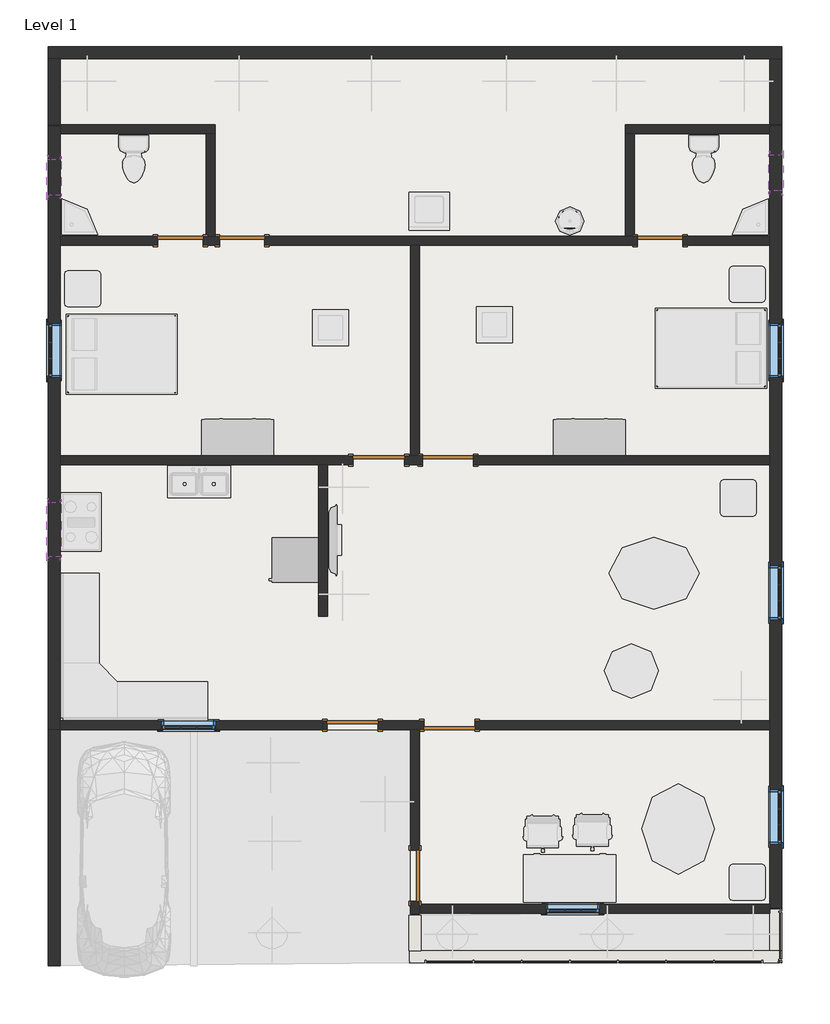
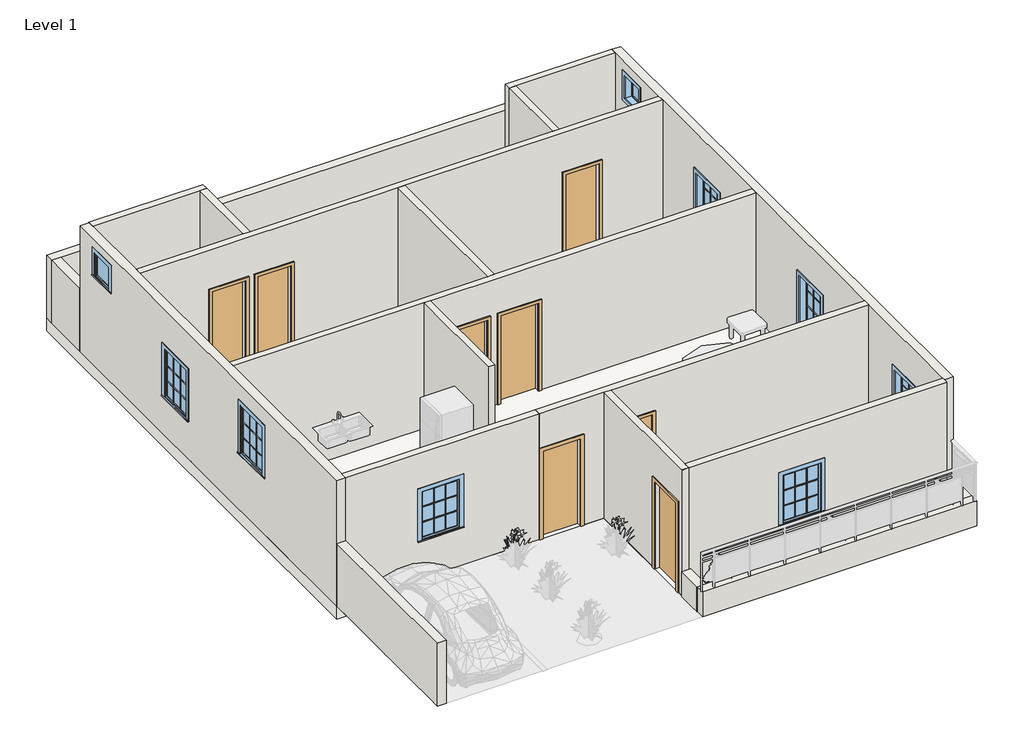
# One storey, part 1 of 2: 21 walls, 9 windows, 8 doors, 1 slab.
"""IFC4 building model written with IfcOpenShell, lengths in millimetres."""

from ifc_helpers import new_model, si_unit, frame, origin, origin_with_axes, place, context, project, spatial, polyline, outline, extrude, faceted_brep, transform, mapped, element, save
from components import door_059fdd7e, door_255cab33, door_b6e9fca3, door_99d96fc5, window_5c190c7e, window_29c06734, window_e41d21a6

model = new_model("IFC4")

# Units and contexts
model_context = context("Model", 3, world=origin())
ifc_project = project(units=[si_unit("LENGTHUNIT", "METRE", prefix="MILLI")], contexts=[model_context])

# Site, building, storey
site = spatial("IfcSite", under=ifc_project)
building = spatial("IfcBuilding", under=site)
storey = spatial("IfcBuildingStorey", under=building, Name="Level 1", Elevation=0.0)

# Doors
placement = place(None, origin())
door_shape = door_059fdd7e(model_context)
element("IfcDoor", 1, ObjectType="Single-Flush : 30\" x 80\"", at=placement, inside=storey, context=model_context, shape_type="MappedRepresentation", body=[
    mapped(door_shape, transform((-10552.7238552, 12812.2234128, 0.0), x_axis=(1.0, 0.0, 0.0), y_axis=(0.0, 1.0, 0.0), z_axis=(0.0, 0.0, 1.0))),
])
door_2_shape = door_255cab33(model_context)
element("IfcDoor", 2, ObjectType="Single-Flush : 30\" x 80\"", at=placement, inside=storey, context=model_context, shape_type="MappedRepresentation", body=[
    mapped(door_2_shape, transform((-9511.3238552, 12812.2234128, 0.0), x_axis=(-1.0, 0.0, 0.0), y_axis=(0.0, -1.0, 0.0), z_axis=(0.0, 0.0, 1.0))),
])
element("IfcDoor", 3, ObjectType="Single-Flush : 30\" x 80\"", at=placement, inside=storey, context=model_context, shape_type="MappedRepresentation", body=[
    mapped(door_2_shape, transform((-2450.1238552, 12812.2234128, 0.0), x_axis=(-1.0, 0.0, 0.0), y_axis=(0.0, -1.0, 0.0), z_axis=(0.0, 0.0, 1.0))),
])
door_3_shape = door_b6e9fca3(model_context)
element("IfcDoor", 4, ObjectType="Single-Flush : 34\" x 84\"", at=placement, inside=storey, context=model_context, shape_type="MappedRepresentation", body=[
    mapped(door_3_shape, transform((-7199.9238552, 9103.8234128, 0.0), x_axis=(1.0, 0.0, 0.0), y_axis=(0.0, 1.0, 0.0), z_axis=(0.0, 0.0, 1.0))),
])
element("IfcDoor", 5, ObjectType="Single-Flush : 34\" x 84\"", at=placement, inside=storey, context=model_context, shape_type="MappedRepresentation", body=[
    mapped(door_3_shape, transform((-6006.1238552, 4633.4234128, 0.0), x_axis=(-1.0, 0.0, 0.0), y_axis=(0.0, -1.0, 0.0), z_axis=(0.0, 0.0, 1.0))),
])
element("IfcDoor", 6, ObjectType="Single-Flush : 34\" x 84\"", at=placement, inside=storey, context=model_context, shape_type="MappedRepresentation", body=[
    mapped(door_3_shape, transform((-6590.3238552, 2093.4234128, 0.0), x_axis=(0.0, -1.0, 0.0), y_axis=(1.0, 0.0, 0.0), z_axis=(0.0, 0.0, 1.0))),
])
door_4_shape = door_99d96fc5(model_context)
element("IfcDoor", 7, ObjectType="Single-Flush : 34\" x 84\"", at=placement, inside=storey, context=model_context, shape_type="MappedRepresentation", body=[
    mapped(door_4_shape, transform((-6031.5238552, 9103.8234128, 0.0), x_axis=(-1.0, 0.0, 0.0), y_axis=(0.0, -1.0, 0.0), z_axis=(0.0, 0.0, 1.0))),
])
element("IfcDoor", 8, ObjectType="Single-Flush : 34\" x 84\"", at=placement, inside=storey, context=model_context, shape_type="MappedRepresentation", body=[
    mapped(door_4_shape, transform((-7644.4238552, 4633.4234128, 0.0), x_axis=(-1.0, 0.0, 0.0), y_axis=(0.0, -1.0, 0.0), z_axis=(0.0, 0.0, 1.0))),
])

# Slab
element("IfcSlab", 9, ObjectType="Generic - 12\"", at=placement, inside=storey, context=model_context, shape_type="SweptSolid", body=[
    extrude(outline(polyline([(-392.7238552, 16088.8234128), (-392.7238552, 1547.3234128), (-392.7238552, 1458.4234128), (-6666.5238552, 1458.4234128), (-6666.5238552, 4557.2234128), (-12787.9238552, 4557.2234128), (-12787.9238552, 16088.8234128), (-392.7238552, 16088.8234128)])), frame((0.0, 0.0, -304.8), z_axis=(0.0, 0.0, 1.0), x_axis=(1.0, 0.0, 0.0)), (0.0, 0.0, 1.0), 304.8),
])

# Walls
element("IfcWall", 10, ObjectType="Generic - 8\"", at=placement, inside=storey, context=model_context, shape_type="Brep", body=[
    faceted_brep([(-12787.9238552, 15885.6234128, 0.0), (-12584.7238552, 15885.6234128, 0.0), (-595.9238552, 15885.6234128, 0.0), (-392.7238552, 15885.6234128, 0.0), (-392.7238552, 15885.6234128, 1524.0), (-595.9238552, 15885.6234128, 1524.0), (-12584.7238552, 15885.6234128, 1524.0), (-12787.9238552, 15885.6234128, 1524.0), (-12787.9238552, 16088.8234128, 0.0), (-12787.9238552, 16088.8234128, 1524.0), (-392.7238552, 16088.8234128, 1524.0), (-392.7238552, 16088.8234128, 0.0)], [[[0, 1, 2, 3, 4, 5, 6, 7]], [[8, 9, 10, 11]], [[3, 2, 1, 0, 8, 11]], [[7, 6, 5, 4, 10, 9]], [[0, 7, 9, 8]], [[4, 3, 11, 10]]]),
])
element("IfcWall", 11, ObjectType="Generic - 8\"", at=placement, inside=storey, context=model_context, shape_type="SweptSolid", body=[
    extrude(outline(polyline([(-12787.9238552, 14768.0234128), (-12787.9238552, 15885.6234128), (-12584.7238552, 15885.6234128), (-12584.7238552, 14768.0234128), (-12787.9238552, 14768.0234128)])), origin_with_axes(), (0.0, 0.0, 1.0), 1524.0),
])
element("IfcWall", 12, ObjectType="Generic - 8\"", at=placement, inside=storey, context=model_context, shape_type="SweptSolid", body=[
    extrude(outline(polyline([(-392.7238552, 1521.9234128), (-392.7238552, 823.4234128), (-595.9238552, 823.4234128), (-595.9238552, 1521.9234128), (-392.7238552, 1521.9234128)])), origin_with_axes(), (0.0, 0.0, 1.0), 609.6),
])
element("IfcWall", 13, ObjectType="Generic - 8\"", at=placement, inside=storey, context=model_context, shape_type="Brep", body=[
    faceted_brep([(-6679.2238552, 620.2234128, 0.0), (-392.7238552, 620.2234128, 0.0), (-392.7238552, 620.2234128, 609.6), (-6679.2238552, 620.2234128, 609.6), (-6679.2238552, 823.4234128, 0.0), (-6679.2238552, 823.4234128, 609.6), (-6488.7238552, 823.4234128, 609.6), (-595.9238552, 823.4234128, 609.6), (-392.7238552, 823.4234128, 609.6), (-392.7238552, 823.4234128, 0.0), (-595.9238552, 823.4234128, 0.0), (-6488.7238552, 823.4234128, 0.0)], [[[0, 1, 2, 3]], [[4, 5, 6, 7, 8, 9, 10, 11]], [[1, 0, 4, 11, 10, 9]], [[3, 2, 8, 7, 6, 5]], [[0, 3, 5, 4]], [[2, 1, 9, 8]]]),
])
element("IfcWall", 14, ObjectType="Generic - 8\"", at=placement, inside=storey, context=model_context, shape_type="Brep", body=[
    faceted_brep([(-6691.9238552, 1420.3234128, 0.0), (-6691.9238552, 823.4234128, 0.0), (-6691.9238552, 823.4234128, 609.6), (-6691.9238552, 1420.3234128, 609.6), (-6488.7238552, 1420.3234128, 0.0), (-6488.7238552, 1420.3234128, 609.6), (-6488.7238552, 823.4234128, 609.6), (-6488.7238552, 823.4234128, 0.0), (-6679.2238552, 823.4234128, 0.0), (-6679.2238552, 823.4234128, 609.6)], [[[0, 1, 2, 3]], [[4, 5, 6, 7]], [[1, 0, 4, 7, 8]], [[3, 2, 9, 6, 5]], [[0, 3, 5, 4]], [[2, 1, 8, 7, 6, 9]]]),
])
element("IfcWall", 15, ObjectType="Generic - 8\"", at=placement, inside=storey, context=model_context, shape_type="SweptSolid", body=[
    extrude(outline(polyline([(-392.7238552, 15885.6234128), (-392.7238552, 14780.7234128), (-595.9238552, 14780.7234128), (-595.9238552, 15885.6234128), (-392.7238552, 15885.6234128)])), origin_with_axes(), (0.0, 0.0, 1.0), 1524.0),
])
element("IfcWall", 16, ObjectType="Generic - 8\"", at=placement, inside=storey, context=model_context, shape_type="SweptSolid", body=[
    extrude(outline(polyline([(-12787.9238552, 569.4234128), (-12787.9238552, 4557.2234128), (-12584.7238552, 4557.2234128), (-12584.7238552, 569.4234128), (-12787.9238552, 569.4234128)])), origin_with_axes(), (0.0, 0.0, 1.0), 1524.0),
])
element("IfcWall", 17, ObjectType="Generic - 8\" 2", at=placement, inside=storey, context=model_context, shape_type="Brep", body=[
    faceted_brep([(-392.7238552, 1547.3234128, 0.0), (-392.7238552, 14755.3234128, 0.0), (-392.7238552, 14755.3234128, 3048.0), (-392.7238552, 1547.3234128, 3048.0), (-392.7238552, 2626.8234128, 2133.6), (-392.7238552, 3541.2234128, 2133.6), (-392.7238552, 3541.2234128, 914.4), (-392.7238552, 2626.8234128, 914.4), (-392.7238552, 6411.4234128, 2133.6), (-392.7238552, 7325.8234128, 2133.6), (-392.7238552, 7325.8234128, 914.4), (-392.7238552, 6411.4234128, 914.4), (-392.7238552, 10500.8234128, 2133.6), (-392.7238552, 11415.2234128, 2133.6), (-392.7238552, 11415.2234128, 914.4), (-392.7238552, 10500.8234128, 914.4), (-392.7238552, 13650.4234128, 2768.6), (-392.7238552, 14260.0234128, 2768.6), (-392.7238552, 14260.0234128, 2159.0), (-392.7238552, 13650.4234128, 2159.0), (-595.9238552, 1547.3234128, 0.0), (-595.9238552, 1547.3234128, 3048.0), (-595.9238552, 1610.8234128, 3048.0), (-595.9238552, 4557.2234128, 3048.0), (-595.9238552, 4709.6234128, 3048.0), (-595.9238552, 9027.6234128, 3048.0), (-595.9238552, 9180.0234128, 3048.0), (-595.9238552, 12736.0234128, 3048.0), (-595.9238552, 12888.4234128, 3048.0), (-595.9238552, 14615.6234128, 3048.0), (-595.9238552, 14755.3234128, 3048.0), (-595.9238552, 14755.3234128, 0.0), (-595.9238552, 14615.6234128, 0.0), (-595.9238552, 12888.4234128, 0.0), (-595.9238552, 12736.0234128, 0.0), (-595.9238552, 9180.0234128, 0.0), (-595.9238552, 9027.6234128, 0.0), (-595.9238552, 4709.6234128, 0.0), (-595.9238552, 4557.2234128, 0.0), (-595.9238552, 1610.8234128, 0.0), (-595.9238552, 2626.8234128, 2133.6), (-595.9238552, 2626.8234128, 914.4), (-595.9238552, 3541.2234128, 914.4), (-595.9238552, 3541.2234128, 2133.6), (-595.9238552, 6411.4234128, 2133.6), (-595.9238552, 6411.4234128, 914.4), (-595.9238552, 7325.8234128, 914.4), (-595.9238552, 7325.8234128, 2133.6), (-595.9238552, 10500.8234128, 2133.6), (-595.9238552, 10500.8234128, 914.4), (-595.9238552, 11415.2234128, 914.4), (-595.9238552, 11415.2234128, 2133.6), (-595.9238552, 13650.4234128, 2768.6), (-595.9238552, 13650.4234128, 2159.0), (-595.9238552, 14260.0234128, 2159.0), (-595.9238552, 14260.0234128, 2768.6)], [[[0, 1, 2, 3], [4, 5, 6, 7], [8, 9, 10, 11], [12, 13, 14, 15], [16, 17, 18, 19]], [[20, 21, 22, 23, 24, 25, 26, 27, 28, 29, 30, 31, 32, 33, 34, 35, 36, 37, 38, 39], [40, 41, 42, 43], [44, 45, 46, 47], [48, 49, 50, 51], [52, 53, 54, 55]], [[1, 0, 20, 39, 38, 37, 36, 35, 34, 33, 32, 31]], [[2, 1, 31, 30]], [[0, 3, 21, 20]], [[41, 40, 4, 7]], [[42, 41, 7, 6]], [[43, 42, 6, 5]], [[40, 43, 5, 4]], [[45, 44, 8, 11]], [[46, 45, 11, 10]], [[47, 46, 10, 9]], [[44, 47, 9, 8]], [[49, 48, 12, 15]], [[50, 49, 15, 14]], [[51, 50, 14, 13]], [[48, 51, 13, 12]], [[53, 52, 16, 19]], [[54, 53, 19, 18]], [[55, 54, 18, 17]], [[52, 55, 17, 16]], [[3, 2, 30, 29, 28, 27, 26, 25, 24, 23, 22, 21]]]),
])
element("IfcWall", 18, ObjectType="Generic - 8\" 2", at=placement, inside=storey, context=model_context, shape_type="Brep", body=[
    faceted_brep([(-12787.9238552, 14742.6234128, 0.0), (-12787.9238552, 4557.2234128, 0.0), (-12787.9238552, 4557.2234128, 3048.0), (-12787.9238552, 14742.6234128, 3048.0), (-12787.9238552, 11415.2234128, 2133.6), (-12787.9238552, 10500.8234128, 2133.6), (-12787.9238552, 10500.8234128, 914.4), (-12787.9238552, 11415.2234128, 914.4), (-12787.9238552, 8392.6234128, 2590.8), (-12787.9238552, 7478.2234128, 2590.8), (-12787.9238552, 7478.2234128, 1371.6), (-12787.9238552, 8392.6234128, 1371.6), (-12787.9238552, 14183.8234128, 2768.6), (-12787.9238552, 13574.2234128, 2768.6), (-12787.9238552, 13574.2234128, 2159.0), (-12787.9238552, 14183.8234128, 2159.0), (-12584.7238552, 14742.6234128, 0.0), (-12584.7238552, 14742.6234128, 3048.0), (-12584.7238552, 14615.6234128, 3048.0), (-12584.7238552, 12888.4234128, 3048.0), (-12584.7238552, 12736.0234128, 3048.0), (-12584.7238552, 9180.0234128, 3048.0), (-12584.7238552, 9027.6234128, 3048.0), (-12584.7238552, 4709.6234128, 3048.0), (-12584.7238552, 4557.2234128, 3048.0), (-12584.7238552, 4557.2234128, 1524.0), (-12584.7238552, 4557.2234128, 0.0), (-12584.7238552, 4709.6234128, 0.0), (-12584.7238552, 9027.6234128, 0.0), (-12584.7238552, 9180.0234128, 0.0), (-12584.7238552, 12736.0234128, 0.0), (-12584.7238552, 12888.4234128, 0.0), (-12584.7238552, 14615.6234128, 0.0), (-12584.7238552, 11415.2234128, 2133.6), (-12584.7238552, 11415.2234128, 914.4), (-12584.7238552, 10500.8234128, 914.4), (-12584.7238552, 10500.8234128, 2133.6), (-12584.7238552, 8392.6234128, 2590.8), (-12584.7238552, 8392.6234128, 1371.6), (-12584.7238552, 7478.2234128, 1371.6), (-12584.7238552, 7478.2234128, 2590.8), (-12584.7238552, 14183.8234128, 2768.6), (-12584.7238552, 14183.8234128, 2159.0), (-12584.7238552, 13574.2234128, 2159.0), (-12584.7238552, 13574.2234128, 2768.6)], [[[0, 1, 2, 3], [4, 5, 6, 7], [8, 9, 10, 11], [12, 13, 14, 15]], [[16, 17, 18, 19, 20, 21, 22, 23, 24, 25, 26, 27, 28, 29, 30, 31, 32], [33, 34, 35, 36], [37, 38, 39, 40], [41, 42, 43, 44]], [[1, 0, 16, 32, 31, 30, 29, 28, 27, 26]], [[2, 1, 26, 25, 24]], [[0, 3, 17, 16]], [[34, 33, 4, 7]], [[35, 34, 7, 6]], [[36, 35, 6, 5]], [[33, 36, 5, 4]], [[38, 37, 8, 11]], [[39, 38, 11, 10]], [[40, 39, 10, 9]], [[37, 40, 9, 8]], [[42, 41, 12, 15]], [[43, 42, 15, 14]], [[44, 43, 14, 13]], [[41, 44, 13, 12]], [[3, 2, 24, 23, 22, 21, 20, 19, 18, 17]]]),
])
element("IfcWall", 19, ObjectType="INNER WALL 6\"", at=placement, inside=storey, context=model_context, shape_type="Brep", body=[
    faceted_brep([(-12584.7238552, 14615.6234128, 0.0), (-10120.9238552, 14615.6234128, 0.0), (-9968.5238552, 14615.6234128, 0.0), (-9968.5238552, 14615.6234128, 3048.0), (-10120.9238552, 14615.6234128, 3048.0), (-12584.7238552, 14615.6234128, 3048.0), (-12584.7238552, 14768.0234128, 0.0), (-12584.7238552, 14768.0234128, 3048.0), (-9968.5238552, 14768.0234128, 3048.0), (-9968.5238552, 14768.0234128, 0.0), (-12584.7238552, 14742.6234128, 0.0), (-12584.7238552, 14742.6234128, 3048.0)], [[[0, 1, 2, 3, 4, 5]], [[6, 7, 8, 9]], [[2, 1, 0, 10, 6, 9]], [[0, 5, 11, 7, 6, 10]], [[3, 2, 9, 8]], [[5, 4, 3, 8, 7, 11]]]),
])
element("IfcWall", 20, ObjectType="INNER WALL 6\"", at=placement, inside=storey, context=model_context, shape_type="SweptSolid", body=[
    extrude(outline(polyline([(-10120.9238552, 12888.4234128), (-10120.9238552, 14615.6234128), (-9968.5238552, 14615.6234128), (-9968.5238552, 12888.4234128), (-10120.9238552, 12888.4234128)])), origin_with_axes(), (0.0, 0.0, 1.0), 3048.0),
])
element("IfcWall", 21, ObjectType="INNER WALL 6\"", at=placement, inside=storey, context=model_context, shape_type="Brep", body=[
    faceted_brep([(-2831.1238552, 12888.4234128, 2032.0), (-2831.1238552, 12888.4234128, 0.0), (-2881.9238552, 12888.4234128, 0.0), (-3034.3238552, 12888.4234128, 0.0), (-9130.3238552, 12888.4234128, 0.0), (-9130.3238552, 12888.4234128, 2032.0), (-9892.3238552, 12888.4234128, 2032.0), (-9892.3238552, 12888.4234128, 0.0), (-9968.5238552, 12888.4234128, 0.0), (-10120.9238552, 12888.4234128, 0.0), (-10171.7238552, 12888.4234128, 0.0), (-10171.7238552, 12888.4234128, 2032.0), (-10933.7238552, 12888.4234128, 2032.0), (-10933.7238552, 12888.4234128, 0.0), (-12584.7238552, 12888.4234128, 0.0), (-12584.7238552, 12888.4234128, 3048.0), (-10120.9238552, 12888.4234128, 3048.0), (-9968.5238552, 12888.4234128, 3048.0), (-3034.3238552, 12888.4234128, 3048.0), (-2881.9238552, 12888.4234128, 3048.0), (-595.9238552, 12888.4234128, 3048.0), (-595.9238552, 12888.4234128, 0.0), (-2069.1238552, 12888.4234128, 0.0), (-2069.1238552, 12888.4234128, 2032.0), (-9130.3238552, 12736.0234128, 0.0), (-6666.5238552, 12736.0234128, 0.0), (-6514.1238552, 12736.0234128, 0.0), (-2831.1238552, 12736.0234128, 0.0), (-2831.1238552, 12736.0234128, 2032.0), (-2069.1238552, 12736.0234128, 2032.0), (-2069.1238552, 12736.0234128, 0.0), (-595.9238552, 12736.0234128, 0.0), (-595.9238552, 12736.0234128, 3048.0), (-6514.1238552, 12736.0234128, 3048.0), (-6666.5238552, 12736.0234128, 3048.0), (-12584.7238552, 12736.0234128, 3048.0), (-12584.7238552, 12736.0234128, 0.0), (-10933.7238552, 12736.0234128, 0.0), (-10933.7238552, 12736.0234128, 2032.0), (-10171.7238552, 12736.0234128, 2032.0), (-10171.7238552, 12736.0234128, 0.0), (-9892.3238552, 12736.0234128, 0.0), (-9892.3238552, 12736.0234128, 2032.0), (-9130.3238552, 12736.0234128, 2032.0)], [[[0, 1, 2, 3, 4, 5, 6, 7, 8, 9, 10, 11, 12, 13, 14, 15, 16, 17, 18, 19, 20, 21, 22, 23]], [[24, 25, 26, 27, 28, 29, 30, 31, 32, 33, 34, 35, 36, 37, 38, 39, 40, 41, 42, 43]], [[37, 36, 14, 13]], [[10, 9, 8, 7, 41, 40]], [[22, 21, 31, 30]], [[4, 3, 2, 1, 27, 26, 25, 24]], [[15, 14, 36, 35]], [[21, 20, 32, 31]], [[11, 10, 40, 39]], [[12, 11, 39, 38]], [[13, 12, 38, 37]], [[42, 41, 7, 6]], [[43, 42, 6, 5]], [[24, 43, 5, 4]], [[28, 27, 1, 0]], [[29, 28, 0, 23]], [[30, 29, 23, 22]], [[20, 19, 18, 17, 16, 15, 35, 34, 33, 32]]]),
])
element("IfcWall", 22, ObjectType="INNER WALL 6\"", at=placement, inside=storey, context=model_context, shape_type="Brep", body=[
    faceted_brep([(-595.9238552, 14768.0234128, 0.0), (-3034.3238552, 14768.0234128, 0.0), (-3034.3238552, 14768.0234128, 3048.0), (-595.9238552, 14768.0234128, 3048.0), (-595.9238552, 14615.6234128, 0.0), (-595.9238552, 14615.6234128, 3048.0), (-2881.9238552, 14615.6234128, 3048.0), (-3034.3238552, 14615.6234128, 3048.0), (-3034.3238552, 14615.6234128, 0.0), (-2881.9238552, 14615.6234128, 0.0), (-595.9238552, 14755.3234128, 0.0), (-595.9238552, 14755.3234128, 3048.0)], [[[0, 1, 2, 3]], [[4, 5, 6, 7, 8, 9]], [[1, 0, 10, 4, 9, 8]], [[2, 1, 8, 7]], [[0, 3, 11, 5, 4, 10]], [[3, 2, 7, 6, 5, 11]]]),
])
element("IfcWall", 23, ObjectType="INNER WALL 6\"", at=placement, inside=storey, context=model_context, shape_type="SweptSolid", body=[
    extrude(outline(polyline([(-3034.3238552, 12888.4234128), (-3034.3238552, 14615.6234128), (-2881.9238552, 14615.6234128), (-2881.9238552, 12888.4234128), (-3034.3238552, 12888.4234128)])), origin_with_axes(), (0.0, 0.0, 1.0), 3048.0),
])
element("IfcWall", 24, ObjectType="INNER WALL 6\"", at=placement, inside=storey, context=model_context, shape_type="SweptSolid", body=[
    extrude(outline(polyline([(-6666.5238552, 9180.0234128), (-6666.5238552, 12736.0234128), (-6514.1238552, 12736.0234128), (-6514.1238552, 9180.0234128), (-6666.5238552, 9180.0234128)])), origin_with_axes(), (0.0, 0.0, 1.0), 3048.0),
])
element("IfcWall", 25, ObjectType="INNER WALL 6\"", at=placement, inside=storey, context=model_context, shape_type="Brep", body=[
    faceted_brep([(-6463.3238552, 9180.0234128, 2133.6), (-6463.3238552, 9180.0234128, 0.0), (-6514.1238552, 9180.0234128, 0.0), (-6666.5238552, 9180.0234128, 0.0), (-6768.1238552, 9180.0234128, 0.0), (-6768.1238552, 9180.0234128, 2133.6), (-7631.7238552, 9180.0234128, 2133.6), (-7631.7238552, 9180.0234128, 0.0), (-12584.7238552, 9180.0234128, 0.0), (-12584.7238552, 9180.0234128, 3048.0), (-6666.5238552, 9180.0234128, 3048.0), (-6514.1238552, 9180.0234128, 3048.0), (-595.9238552, 9180.0234128, 3048.0), (-595.9238552, 9180.0234128, 0.0), (-5599.7238552, 9180.0234128, 0.0), (-5599.7238552, 9180.0234128, 2133.6), (-6768.1238552, 9027.6234128, 0.0), (-6463.3238552, 9027.6234128, 0.0), (-6463.3238552, 9027.6234128, 2133.6), (-5599.7238552, 9027.6234128, 2133.6), (-5599.7238552, 9027.6234128, 0.0), (-595.9238552, 9027.6234128, 0.0), (-595.9238552, 9027.6234128, 3048.0), (-8063.5238552, 9027.6234128, 3048.0), (-8215.9238552, 9027.6234128, 3048.0), (-12584.7238552, 9027.6234128, 3048.0), (-12584.7238552, 9027.6234128, 0.0), (-8215.9238552, 9027.6234128, 0.0), (-8063.5238552, 9027.6234128, 0.0), (-7631.7238552, 9027.6234128, 0.0), (-7631.7238552, 9027.6234128, 2133.6), (-6768.1238552, 9027.6234128, 2133.6)], [[[0, 1, 2, 3, 4, 5, 6, 7, 8, 9, 10, 11, 12, 13, 14, 15]], [[16, 17, 18, 19, 20, 21, 22, 23, 24, 25, 26, 27, 28, 29, 30, 31]], [[29, 28, 27, 26, 8, 7]], [[14, 13, 21, 20]], [[4, 3, 2, 1, 17, 16]], [[9, 8, 26, 25]], [[13, 12, 22, 21]], [[5, 4, 16, 31]], [[6, 5, 31, 30]], [[7, 6, 30, 29]], [[18, 17, 1, 0]], [[19, 18, 0, 15]], [[20, 19, 15, 14]], [[12, 11, 10, 9, 25, 24, 23, 22]]]),
])
element("IfcWall", 26, ObjectType="INNER WALL 6\"", at=placement, inside=storey, context=model_context, shape_type="SweptSolid", body=[
    extrude(outline(polyline([(-8215.9238552, 6474.9234128), (-8215.9238552, 9027.6234128), (-8063.5238552, 9027.6234128), (-8063.5238552, 6474.9234128), (-8215.9238552, 6474.9234128)])), origin_with_axes(), (0.0, 0.0, 1.0), 3048.0),
])
element("IfcWall", 27, ObjectType="INNER WALL 6\"", at=placement, inside=storey, context=model_context, shape_type="Brep", body=[
    faceted_brep([(-6666.5238552, 1661.6234128, 2133.6), (-6666.5238552, 1661.6234128, 0.0), (-6666.5238552, 1445.7234128, 0.0), (-6666.5238552, 1445.7234128, 3048.0), (-6666.5238552, 1458.4234128, 3048.0), (-6666.5238552, 4557.2234128, 3048.0), (-6666.5238552, 4557.2234128, 0.0), (-6666.5238552, 2525.2234128, 0.0), (-6666.5238552, 2525.2234128, 2133.6), (-6514.1238552, 1445.7234128, 0.0), (-6514.1238552, 1458.4234128, 0.0), (-6514.1238552, 1610.8234128, 0.0), (-6514.1238552, 1661.6234128, 0.0), (-6514.1238552, 1661.6234128, 2133.6), (-6514.1238552, 2525.2234128, 2133.6), (-6514.1238552, 2525.2234128, 0.0), (-6514.1238552, 4557.2234128, 0.0), (-6514.1238552, 4557.2234128, 3048.0), (-6514.1238552, 1610.8234128, 3048.0), (-6514.1238552, 1458.4234128, 3048.0), (-6514.1238552, 1445.7234128, 3048.0)], [[[0, 1, 2, 3, 4, 5, 6, 7, 8]], [[9, 10, 11, 12, 13, 14, 15, 16, 17, 18, 19, 20]], [[7, 6, 16, 15]], [[2, 1, 12, 11, 10, 9]], [[3, 2, 9, 20]], [[6, 5, 17, 16]], [[13, 12, 1, 0]], [[14, 13, 0, 8]], [[15, 14, 8, 7]], [[4, 3, 20, 19]], [[5, 4, 19, 18, 17]]]),
])
element("IfcWall", 28, ObjectType="INNER WALL 6\"", at=placement, inside=storey, context=model_context, shape_type="Brep", body=[
    faceted_brep([(-6514.1238552, 1458.4234128, 0.0), (-595.9238552, 1458.4234128, 0.0), (-595.9238552, 1458.4234128, 3048.0), (-6514.1238552, 1458.4234128, 3048.0), (-4380.5238552, 1458.4234128, 2133.6), (-3466.1238552, 1458.4234128, 2133.6), (-3466.1238552, 1458.4234128, 914.4), (-4380.5238552, 1458.4234128, 914.4), (-6514.1238552, 1610.8234128, 0.0), (-6514.1238552, 1610.8234128, 3048.0), (-595.9238552, 1610.8234128, 3048.0), (-595.9238552, 1610.8234128, 0.0), (-4380.5238552, 1610.8234128, 2133.6), (-4380.5238552, 1610.8234128, 914.4), (-3466.1238552, 1610.8234128, 914.4), (-3466.1238552, 1610.8234128, 2133.6), (-595.9238552, 1547.3234128, 0.0), (-595.9238552, 1547.3234128, 3048.0)], [[[0, 1, 2, 3], [4, 5, 6, 7]], [[8, 9, 10, 11], [12, 13, 14, 15]], [[1, 0, 8, 11, 16]], [[2, 1, 16, 11, 10, 17]], [[0, 3, 9, 8]], [[13, 12, 4, 7]], [[14, 13, 7, 6]], [[15, 14, 6, 5]], [[12, 15, 5, 4]], [[3, 2, 17, 10, 9]]]),
])
element("IfcWall", 29, ObjectType="INNER WALL 6\"", at=placement, inside=storey, context=model_context, shape_type="SweptSolid", body=[
    extrude(outline(polyline([(0.0, -8152.4238552), (3048.0, -8152.4238552), (3048.0, -12584.7238552), (0.0, -12584.7238552), (0.0, -8152.4238552)]), holes=[polyline([(2133.6, -10870.2238552), (2133.6, -9955.8238552), (914.4, -9955.8238552), (914.4, -10870.2238552), (2133.6, -10870.2238552)])]), frame((0.0, 4557.2234128, 0.0), z_axis=(0.0, 1.0, 0.0), x_axis=(0.0, 0.0, 1.0)), (0.0, 0.0, 1.0), 152.4),
])
element("IfcWall", 30, ObjectType="INNER WALL 6\"", at=placement, inside=storey, context=model_context, shape_type="Brep", body=[
    faceted_brep([(-7212.6238552, 4557.2234128, 0.0), (-6666.5238552, 4557.2234128, 0.0), (-6514.1238552, 4557.2234128, 0.0), (-6437.9238552, 4557.2234128, 0.0), (-6437.9238552, 4557.2234128, 2133.6), (-5574.3238552, 4557.2234128, 2133.6), (-5574.3238552, 4557.2234128, 0.0), (-595.9238552, 4557.2234128, 0.0), (-595.9238552, 4557.2234128, 3048.0), (-6514.1238552, 4557.2234128, 3048.0), (-6666.5238552, 4557.2234128, 3048.0), (-8152.4238552, 4557.2234128, 3048.0), (-8152.4238552, 4557.2234128, 0.0), (-8076.2238552, 4557.2234128, 0.0), (-8076.2238552, 4557.2234128, 2133.6), (-7212.6238552, 4557.2234128, 2133.6), (-6437.9238552, 4709.6234128, 2133.6), (-6437.9238552, 4709.6234128, 0.0), (-7212.6238552, 4709.6234128, 0.0), (-7212.6238552, 4709.6234128, 2133.6), (-8076.2238552, 4709.6234128, 2133.6), (-8076.2238552, 4709.6234128, 0.0), (-8152.4238552, 4709.6234128, 0.0), (-8152.4238552, 4709.6234128, 3048.0), (-595.9238552, 4709.6234128, 3048.0), (-595.9238552, 4709.6234128, 0.0), (-5574.3238552, 4709.6234128, 0.0), (-5574.3238552, 4709.6234128, 2133.6)], [[[0, 1, 2, 3, 4, 5, 6, 7, 8, 9, 10, 11, 12, 13, 14, 15]], [[16, 17, 18, 19, 20, 21, 22, 23, 24, 25, 26, 27]], [[22, 21, 13, 12]], [[26, 25, 7, 6]], [[18, 17, 3, 2, 1, 0]], [[12, 11, 23, 22]], [[8, 7, 25, 24]], [[14, 13, 21, 20]], [[15, 14, 20, 19]], [[0, 15, 19, 18]], [[4, 3, 17, 16]], [[5, 4, 16, 27]], [[6, 5, 27, 26]], [[11, 10, 9, 8, 24, 23]]]),
])

# Windows
window_shape = window_5c190c7e(model_context)
element("IfcWindow", 31, ObjectType="Casement 3x3 with Trim : 36\" x 48\"", at=placement, inside=storey, context=model_context, shape_type="MappedRepresentation", body=[
    mapped(window_shape, transform((-10413.0238552, 4633.4234128, 0.0), x_axis=(-1.0, 0.0, 0.0), y_axis=(0.0, -1.0, 0.0), z_axis=(0.0, 0.0, 1.0))),
])
element("IfcWindow", 32, ObjectType="Casement 3x3 with Trim : 36\" x 48\"", at=placement, inside=storey, context=model_context, shape_type="MappedRepresentation", body=[
    mapped(window_shape, transform((-3923.3238552, 1534.6234128, 0.0), x_axis=(-1.0, 0.0, 0.0), y_axis=(0.0, -1.0, 0.0), z_axis=(0.0, 0.0, 1.0))),
])
window_2_shape = window_29c06734(model_context)
element("IfcWindow", 33, ObjectType="Casement 3x3 with Trim : 36\" x 48\"", at=placement, inside=storey, context=model_context, shape_type="MappedRepresentation", body=[
    mapped(window_2_shape, transform((-12686.3238552, 10958.0234128, 0.0), x_axis=(0.0, 1.0, 0.0), y_axis=(-1.0, 0.0, 0.0), z_axis=(0.0, 0.0, 1.0))),
])
element("IfcWindow", 34, ObjectType="Casement 3x3 with Trim : 36\" x 48\"", at=placement, inside=storey, context=model_context, shape_type="MappedRepresentation", body=[
    mapped(window_2_shape, transform((-12686.3238552, 7935.4234128, 457.2), x_axis=(0.0, 1.0, 0.0), y_axis=(-1.0, 0.0, 0.0), z_axis=(0.0, 0.0, 1.0))),
])
element("IfcWindow", 35, ObjectType="Casement 3x3 with Trim : 36\" x 48\"", at=placement, inside=storey, context=model_context, shape_type="MappedRepresentation", body=[
    mapped(window_2_shape, transform((-494.3238552, 3084.0234128, 0.0), x_axis=(0.0, -1.0, 0.0), y_axis=(1.0, 0.0, 0.0), z_axis=(0.0, 0.0, 1.0))),
])
element("IfcWindow", 36, ObjectType="Casement 3x3 with Trim : 36\" x 48\"", at=placement, inside=storey, context=model_context, shape_type="MappedRepresentation", body=[
    mapped(window_2_shape, transform((-494.3238552, 6868.6234128, 0.0), x_axis=(0.0, -1.0, 0.0), y_axis=(1.0, 0.0, 0.0), z_axis=(0.0, 0.0, 1.0))),
])
element("IfcWindow", 37, ObjectType="Casement 3x3 with Trim : 36\" x 48\"", at=placement, inside=storey, context=model_context, shape_type="MappedRepresentation", body=[
    mapped(window_2_shape, transform((-494.3238552, 10958.0234128, 0.0), x_axis=(0.0, -1.0, 0.0), y_axis=(1.0, 0.0, 0.0), z_axis=(0.0, 0.0, 1.0))),
])
window_3_shape = window_e41d21a6(model_context)
element("IfcWindow", 38, ObjectType="Transom with Trim : 24\" x 24\"", at=placement, inside=storey, context=model_context, shape_type="MappedRepresentation", body=[
    mapped(window_3_shape, transform((-494.3238552, 13917.1234128, 0.0), x_axis=(0.0, -1.0, 0.0), y_axis=(1.0, 0.0, 0.0), z_axis=(0.0, 0.0, 1.0))),
])
element("IfcWindow", 39, ObjectType="Transom with Trim : 24\" x 24\"", at=placement, inside=storey, context=model_context, shape_type="MappedRepresentation", body=[
    mapped(window_3_shape, transform((-12686.3238552, 13917.1234128, 0.0), x_axis=(0.0, 1.0, 0.0), y_axis=(-1.0, 0.0, 0.0), z_axis=(0.0, 0.0, 1.0))),
])

save(model, "model.ifc")

# Revit data of these elements
# Type "Single-Flush : 30\" x 80\""
#   Type Mark = "5"
#   Construction Type Id = "MDOOR"
#   Assembly Code = "C1020"
#   Analytic Construction = "Metal"
#   Thickness = 0' - 2"
#   Heat Transfer Coefficient (U) = 0.651978 BTU/(h·ft²·°F)
#   Height = 6' - 8"
#   Trim Projection Ext = 0' - 1"
#   Trim Projection Int = 0' - 1"
#   Trim Width = 0' - 3"
#   Width = 2' - 6"
#   Define Thermal Properties by = 1
#   Door Material = Door - Panel
#   Frame Material = Door - Frame
#   Visual Light Transmittance = 0
#   Solar Heat Gain Coefficient = 0
#   Function = (empty or 0)
#   Wall Closure = (empty or 0)
# Type "Single-Flush : 34\" x 84\""
#   Type Mark = "2"
#   Construction Type Id = "MDOOR"
#   Assembly Code = "C1020"
#   Analytic Construction = "Metal"
#   Thickness = 0' - 2"
#   Heat Transfer Coefficient (U) = 0.651978 BTU/(h·ft²·°F)
#   Height = 7' - 0"
#   Trim Projection Ext = 0' - 1"
#   Trim Projection Int = 0' - 1"
#   Trim Width = 0' - 3"
#   Width = 2' - 10"
#   Define Thermal Properties by = 1
#   Door Material = Door - Panel
#   Frame Material = Door - Frame
#   Visual Light Transmittance = 0
#   Solar Heat Gain Coefficient = 0
#   Function = (empty or 0)
#   Wall Closure = (empty or 0)
# Type "Generic - 12\""
#   Assembly Code = "B1010"
#   Function = 0
#   Layers, outside or top first: 1' - 0" no material (function 1)
# Type "Generic - 8\""
#   Assembly Code = "B2010"
#   Layers, outside or top first: 0' - 8" "Birch" (function 1)
# Type "Generic - 8\" 2"
#   Assembly Code = "B2010"
#   Layers, outside or top first: 0' - 8" "Brick, Common" (function 1)
# Type "INNER WALL 6\""
#   Assembly Code = "B2010"
#   Layers, outside or top first: 0' - 6" "Brick, Common" (function 1)
# Type "Casement 3x3 with Trim : 36\" x 48\""
#   Type Mark = "10"
#   Construction Type Id = "GSP4R"
#   Assembly Code = "B2020100"
#   Analytic Construction = "1/8 in Pilkington single glazing"
#   Visual Light Transmittance = 0.9
#   Solar Heat Gain Coefficient = 0.78
#   Heat Transfer Coefficient (U) = 0.6496 BTU/(h·ft²·°F)
#   Height = 4' - 0"
#   Default Sill Height = 3' - 0"
#   Trim Projection - Ext. = 0' - 0 1/2"
#   Trim Projection - Int. = 0' - 0 3/4"
#   Trim Width - Exterior = 0' - 3 1/2"
#   Trim Width - Interior = 0' - 3 1/2"
#   Width = 3' - 0"
#   Window Inset = 0' - 0 3/4"
#   Define Thermal Properties by = 1
#   Glass Pane Material = Glass
#   Sash Material = Sash
#   Trim Exterior Material = Trim
#   Trim Interior Material = Trim
#   Wall Closure = (empty or 0)
# Type "Transom with Trim : 24\" x 24\""
#   Type Mark = "13"
#   Construction Type Id = "GSP4R"
#   Assembly Code = "B2020100"
#   Analytic Construction = "1/8 in Pilkington single glazing"
#   Visual Light Transmittance = 0.9
#   Solar Heat Gain Coefficient = 0.78
#   Heat Transfer Coefficient (U) = 0.6496 BTU/(h·ft²·°F)
#   Height = 2' - 0"
#   Default Sill Height = 7' - 1"
#   Trim Projection - Ext. = 0' - 0 1/2"
#   Trim Projection - Int. = 0' - 0 3/4"
#   Trim Width - Exterior = 0' - 3 1/2"
#   Trim Width - Interior = 0' - 3 1/2"
#   Width = 2' - 0"
#   Window Inset = 0' - 0 3/4"
#   Define Thermal Properties by = 1
#   Glass Pane Material = Glass
#   Sash Material = Sash
#   Trim Exterior Material = Trim
#   Trim Interior Material = Trim
#   Wall Closure = (empty or 0)
# Elements 1, 2, 3 (IfcDoor, "Single-Flush : 30\" x 80\"")
#   Phase Created = New Construction
#   Materials on its faces: "Door - Frame", "Door - Panel"
# Elements 4, 5, 6, 7, 8 (IfcDoor, "Single-Flush : 34\" x 84\"")
#   Phase Created = New Construction
#   Materials on its faces: "Door - Frame", "Door - Panel"
# Element 9 (IfcSlab, "Generic - 12\"")
#   Height Offset From Level = 0' - 0"
#   Phase Created = New Construction
#   Materials on its faces: "Default Floor"
# Elements 10, 11, 15, 16 (IfcWall, "Generic - 8\"")
#   Top Offset = 0' - 0"
#   Base Offset = 0' - 0"
#   Unconnected Height = 5' - 0"
#   wall height = 5' - 0"
#   Phase Created = New Construction
#   Base Constraint = Level 1
#   Materials on its faces: "Birch"
# Elements 12, 13, 14 (IfcWall, "Generic - 8\"")
#   Top Offset = 0' - 0"
#   Base Offset = 0' - 0"
#   Unconnected Height = 2' - 0"
#   wall height = 2' - 0"
#   Phase Created = New Construction
#   Base Constraint = Level 1
#   Materials on its faces: "Birch"
# Elements 17, 18 (IfcWall, "Generic - 8\" 2")
#   Top Offset = 0' - 0"
#   Base Offset = 0' - 0"
#   Unconnected Height = 10' - 0"
#   wall height = 10' - 0"
#   Phase Created = New Construction
#   Base Constraint = Level 1
#   Materials on its faces: "Brick, Common"
# Elements 19, 20, 21, 22, 23, 24, 25, 26, 27, 28, 29, 30 (IfcWall, "INNER WALL 6\"")
#   Top Offset = 0' - 0"
#   Base Offset = 0' - 0"
#   Unconnected Height = 10' - 0"
#   wall height = 10' - 0"
#   Phase Created = New Construction
#   Base Constraint = Level 1
#   Materials on its faces: "Brick, Common"
# Element 31 (IfcWindow, "Casement 3x3 with Trim : 36\" x 48\"")
#   Mark = "3"
#   Phase Created = New Construction
#   Materials on its faces: "Sash", "Glass", "Trim"
# Element 32 (IfcWindow, "Casement 3x3 with Trim : 36\" x 48\"")
#   Mark = "4"
#   Phase Created = New Construction
#   Materials on its faces: "Sash", "Glass", "Trim"
# Element 33 (IfcWindow, "Casement 3x3 with Trim : 36\" x 48\"")
#   Mark = "1"
#   Phase Created = New Construction
#   Materials on its faces: "Sash", "Glass", "Trim"
# Element 34 (IfcWindow, "Casement 3x3 with Trim : 36\" x 48\"")
#   Mark = "2"
#   Phase Created = New Construction
#   Materials on its faces: "Sash", "Glass", "Trim"
# Element 35 (IfcWindow, "Casement 3x3 with Trim : 36\" x 48\"")
#   Mark = "5"
#   Phase Created = New Construction
#   Materials on its faces: "Sash", "Glass", "Trim"
# Element 36 (IfcWindow, "Casement 3x3 with Trim : 36\" x 48\"")
#   Mark = "6"
#   Phase Created = New Construction
#   Materials on its faces: "Sash", "Glass", "Trim"
# Element 37 (IfcWindow, "Casement 3x3 with Trim : 36\" x 48\"")
#   Mark = "7"
#   Phase Created = New Construction
#   Materials on its faces: "Sash", "Glass", "Trim"
# Element 38 (IfcWindow, "Transom with Trim : 24\" x 24\"")
#   Mark = "8"
#   Phase Created = New Construction
#   Materials on its faces: "Sash", "Trim", "Glass"
# Element 39 (IfcWindow, "Transom with Trim : 24\" x 24\"")
#   Mark = "9"
#   Phase Created = New Construction
#   Materials on its faces: "Sash", "Trim", "Glass"
# Materials
#   "Door - Panel": class "Wood", colour RGB 210 159 95, transparency 0
#   "Door - Frame": colour RGB 118 70 51, transparency 0
#   "Birch": class "Wood", colour RGB 224 178 126, transparency 0, Description = "Betula Alleghaniensis", Cost = 0
#   "Brick, Common": class "Masonry", colour RGB 170 98 104, transparency 0, Description = "Common brick", Cost = 0
#   "Glass": class "Glass", colour RGB 0 128 192, transparency 0.75, Description = "Soda Lime Glass", Cost = 0
#   "Sash": class "Wood", colour RGB 224 178 126, transparency 0
#   "Trim": class "Wood", colour RGB 224 178 126, transparency 0
#   "Default Floor": colour RGB 128 128 128, transparency 0
# Room at (-3799.555, 10959.309) mm, phase "New Construction", upper level "Level 1", upper offset 10' - 0", lower offset 0' - 0"
#   Number = "5"
#   Name = "BEDROOM"
# Room at (-4868.259, 6903.28) mm, phase "New Construction", upper level "Level 1", upper offset 10' - 0", lower offset 0' - 0"
#   Number = "7"
#   Name = "LOUNGE/LIVING"
# Room at (-6501.492, 14640.456) mm, phase "New Construction", upper level "Level 1", upper offset 10' - 0", lower offset 0' - 0"
#   Number = "1"
#   Name = "OPEN AREA"
# Room at (-11537.58, 13746.367) mm, phase "New Construction", upper level "Level 1", upper offset 10' - 0", lower offset 0' - 0"
#   Number = "2"
# Room at (-1757.351, 14001.821) mm, phase "New Construction", upper level "Level 1", upper offset 10' - 0", lower offset 0' - 0"
#   Number = "3"
# Room at (-10260.641, 6716.694) mm, phase "New Construction", upper level "Level 1", upper offset 10' - 0", lower offset 0' - 0"
#   Number = "6"
#   Name = "KITCHEN"
# Room at (-11537.58, 2130.2) mm, phase "New Construction", upper level "Level 1", upper offset 10' - 0", lower offset 0' - 0"
#   Number = "8"
#   Name = "PARKING"
# Room at (-3874.467, 3392.355) mm, phase "New Construction", upper level "Level 1", upper offset 10' - 0", lower offset 0' - 0"
#   Number = "9"
#   Name = "DRAWING"
# Room at (-3586.151, 868.044) mm, phase "New Construction", upper level "Level 1", upper offset 10' - 0", lower offset 0' - 0"
#   Number = "10"
#   Name = "OPEN"
# Room at (-9708.78, 10959.309) mm, phase "New Construction", upper level "Level 1", upper offset 10' - 0", lower offset 0' - 0"
#   Number = "4"
#   Name = "BEDROOM"
